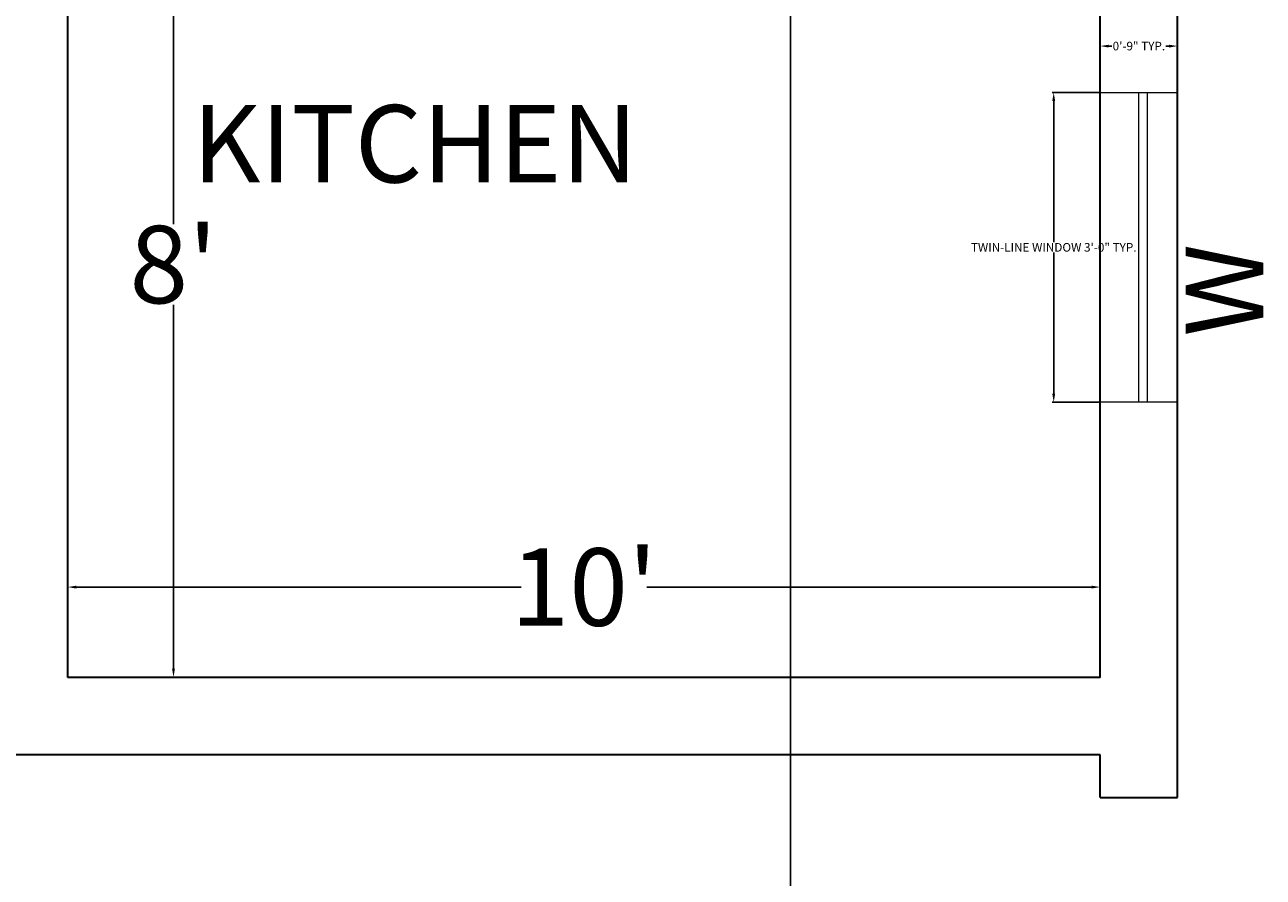
# Model space of a CAD drawing. Units: inches. Extents: x -2189 to 546, y 945 to 2684.
# Tile 6 of 10: x -492 to -348, y 2267 to 2366. Entities that reach past the tile are written whole.
import ezdxf

# ---------------------------------------------------------------- set-up
doc = ezdxf.new("R2010")
doc.units = ezdxf.units.IN
doc.header["$MEASUREMENT"] = 0
for name, color, linetype, lineweight in [('A-ANNO-DIMS', 2, 'Continuous', 13), ('A-ANNO-TEXT', 7, 'Continuous', 18), ('A-AREA-IDEN', 3, 'Continuous', 18), ('A-GLAZ', 4, 'Continuous', 18), ('A-WALL', 7, 'Continuous', 35)]:
    doc.layers.add(name, color=color, linetype=linetype, lineweight=lineweight)
doc.styles.get("Standard").update_dxf_attribs({"font": 'arial.ttf'})
doc.dimstyles.get("Standard").update_dxf_attribs({"dimtxt": 1, "dimasz": 1, "dimexe": 0.18, "dimexo": 0.0625, "dimgap": 0.09, "dimtad": 0, "dimtih": 1, "dimtoh": 1, "dimdec": 0, "dimzin": 0, "dimdsep": 46, "dimlunit": 3, "dimtxsty": 'Standard', "dimcen": 0.09, "dimadec": 0, "dimazin": 0, "dimtfac": 1, "dimtdec": 0, "dimtofl": 0, "dimtmove": 0, "dimatfit": 3, "dimfxl": 1, "dimtolj": 1, "dimtzin": 0, "dimarcsym": 0})

# ---------------------------------------------------------------- blocks, each defined once
blk = doc.blocks.new('*D70')
at = {"layer": 'A-ANNO-DIMS', "color": 0, "lineweight": -2, "transparency": 16777216}
for p, q in [((-486.72, 2386.17), (-474.31, 2386.17)), ((-474.49, 2385.17), (-474.49, 2342.86)), ((-474.49, 2291.17), (-474.49, 2333.49)), ((-486.72, 2290.17), (-474.31, 2290.17))]:
    blk.add_line(p, q, dxfattribs=at)
at = {"layer": 'A-ANNO-DIMS', "color": 0, "transparency": 16777216}
for points in [[(-474.66, 2385.17), (-474.33, 2385.17), (-474.49, 2386.17)], [(-474.66, 2291.17), (-474.33, 2291.17), (-474.49, 2290.17)]]:
    blk.add_solid(points, dxfattribs=at)
at = {"layer": 'Defpoints', "color": 0, "transparency": 16777216}
for p in [(-486.78, 2386.17), (-486.78, 2290.17), (-474.49, 2290.17)]:
    blk.add_point(p, dxfattribs=at)
at = {"layer": 'A-ANNO-DIMS', "color": 0, "transparency": 16777216, "insert": (-474.49, 2338.17), "char_height": 1, "attachment_point": 5}
blk.add_mtext("\\A1;{\\H9x;8'}", dxfattribs=at)
blk = doc.blocks.new('*D71')
at = {"layer": 'A-ANNO-DIMS', "color": 0, "lineweight": -2, "transparency": 16777216}
for p, q in [((-486.78, 2290.24), (-486.78, 2300.85)), ((-485.78, 2300.67), (-434.08, 2300.67)), ((-367.78, 2300.67), (-419.48, 2300.67)), ((-366.78, 2290.24), (-366.78, 2300.85))]:
    blk.add_line(p, q, dxfattribs=at)
at = {"layer": 'A-ANNO-DIMS', "color": 0, "transparency": 16777216}
for points in [[(-485.78, 2300.84), (-485.78, 2300.5), (-486.78, 2300.67)], [(-367.78, 2300.84), (-367.78, 2300.5), (-366.78, 2300.67)]]:
    blk.add_solid(points, dxfattribs=at)
at = {"layer": 'Defpoints', "color": 0, "transparency": 16777216}
for p in [(-366.78, 2300.67), (-486.78, 2290.17), (-366.78, 2290.17)]:
    blk.add_point(p, dxfattribs=at)
at = {"layer": 'A-ANNO-DIMS', "color": 0, "transparency": 16777216, "insert": (-426.78, 2300.67), "char_height": 1, "attachment_point": 5}
blk.add_mtext("\\A1;{\\H9x;10'}", dxfattribs=at)
blk = doc.blocks.new('WIN-36X9-TWINLINE')
for p, q in [((4.5, 0), (4.5, 36)), ((5.5, 0), (5.5, 36))]:
    blk.add_line(p, q)
blk.add_lwpolyline([(9, 0), (0, 0), (0, 36), (9, 36)], close=True)
blk = doc.blocks.new('*D93')
at = {"layer": 'A-ANNO-DIMS', "color": 0, "lineweight": -2, "transparency": 16777216}
for p, q in [((-366.84, 2358.17), (-372.36, 2358.17)), ((-372.18, 2357.17), (-372.18, 2340.78)), ((-372.18, 2323.17), (-372.18, 2339.56)), ((-366.84, 2322.17), (-372.36, 2322.17))]:
    blk.add_line(p, q, dxfattribs=at)
at = {"layer": 'A-ANNO-DIMS', "color": 0, "transparency": 16777216}
for points in [[(-372.35, 2357.17), (-372.01, 2357.17), (-372.18, 2358.17)], [(-372.35, 2323.17), (-372.01, 2323.17), (-372.18, 2322.17)]]:
    blk.add_solid(points, dxfattribs=at)
at = {"layer": 'Defpoints', "color": 0, "transparency": 16777216}
for p in [(-372.18, 2358.17), (-366.78, 2358.17), (-366.78, 2322.17)]:
    blk.add_point(p, dxfattribs=at)
at = {"layer": 'A-ANNO-DIMS', "color": 0, "transparency": 16777216, "insert": (-372.18, 2340.17), "char_height": 1, "attachment_point": 5}
blk.add_mtext('\\A1;TWIN-LINE WINDOW 3\'-0" TYP.', dxfattribs=at)
blk = doc.blocks.new('*D94')
at = {"layer": 'A-ANNO-DIMS', "color": 0, "lineweight": -2, "transparency": 16777216}
for p, q in [((-366.78, 2358.23), (-366.78, 2363.75)), ((-357.78, 2358.23), (-357.78, 2363.75)), ((-365.78, 2363.57), (-365.42, 2363.57)), ((-358.78, 2363.57), (-359.14, 2363.57))]:
    blk.add_line(p, q, dxfattribs=at)
at = {"layer": 'A-ANNO-DIMS', "color": 0, "transparency": 16777216}
for points in [[(-365.78, 2363.73), (-365.78, 2363.4), (-366.78, 2363.57)], [(-358.78, 2363.73), (-358.78, 2363.4), (-357.78, 2363.57)]]:
    blk.add_solid(points, dxfattribs=at)
at = {"layer": 'Defpoints', "color": 0, "transparency": 16777216}
for p in [(-357.78, 2363.57), (-366.78, 2358.17), (-357.78, 2358.17)]:
    blk.add_point(p, dxfattribs=at)
at = {"layer": 'A-ANNO-DIMS', "color": 0, "transparency": 16777216, "insert": (-362.28, 2363.57), "char_height": 1, "attachment_point": 5}
blk.add_mtext('\\A1;0\'-9" TYP.', dxfattribs=at)
blk = doc.blocks.new('*D104')
at = {"layer": 'A-ANNO-DIMS', "color": 0, "lineweight": -2, "transparency": 16777216}
for p, q in [((-493.78, 1873.24), (-493.78, 2683.65)), ((-492.78, 2683.47), (-449.69, 2683.47)), ((-403.78, 2683.47), (-446.86, 2683.47)), ((-402.78, 1873.24), (-402.78, 2683.65))]:
    blk.add_line(p, q, dxfattribs=at)
at = {"layer": 'A-ANNO-DIMS', "color": 0, "transparency": 16777216}
for points in [[(-492.78, 2683.64), (-492.78, 2683.31), (-493.78, 2683.47)], [(-403.78, 2683.64), (-403.78, 2683.31), (-402.78, 2683.47)]]:
    blk.add_solid(points, dxfattribs=at)
at = {"layer": 'Defpoints', "color": 0, "transparency": 16777216}
for p in [(-402.78, 2683.47), (-493.78, 1873.17), (-402.78, 1873.17)]:
    blk.add_point(p, dxfattribs=at)
at = {"layer": 'A-ANNO-DIMS', "color": 0, "transparency": 16777216, "insert": (-448.28, 2683.47), "char_height": 1, "attachment_point": 5}
blk.add_mtext('\\A1;7\'-7"', dxfattribs=at)

msp = doc.modelspace()

# ---------------------------------------------------------------- linework, layer by layer
at = {"layer": 'A-WALL'}
for p, q in [((-357.78, 2276.2), (-357.78, 2446.17)), ((-486.78, 2290.17), (-486.78, 2386.17)), ((-366.78, 2290.17), (-366.78, 2386.17)), ((-366.78, 2290.17), (-486.78, 2290.17)), ((-366.78, 2281.17), (-690.78, 2281.17)), ((-366.78, 2276.2), (-366.78, 2281.17)), ((-366.78, 2276.2), (-357.78, 2276.2))]:
    msp.add_line(p, q, dxfattribs=at)

# ---------------------------------------------------------------- block references
at = {"layer": 'A-GLAZ'}
msp.add_blockref('WIN-36X9-TWINLINE', (-366.78, 2322.17), dxfattribs=at)

# ---------------------------------------------------------------- texts
at = {"layer": 'A-ANNO-TEXT', "insert": (-356.83, 2329.79), "char_height": 9, "attachment_point": 1, "rotation": 90}
msp.add_mtext_dynamic_manual_height_columns('W', width=11.3125, gutter_width=1, heights=[0], dxfattribs=at)
at = {"layer": 'A-AREA-IDEN', "insert": (-472.3, 2356.71), "char_height": 9, "attachment_point": 1}
msp.add_mtext_dynamic_manual_height_columns('KITCHEN', width=69.371, gutter_width=1, heights=[0], dxfattribs=at)

# ---------------------------------------------------------------- dimensions: what is measured, and where the dimension line sits
at = {"layer": 'A-ANNO-DIMS'}
dim = msp.add_linear_dim(base=(-402.78, 2683.47), p1=(-493.78, 1873.17), p2=(-402.78, 1873.17), dimstyle='Standard', override={"dimdec": 1, "dimlfac": 1, "dimrnd": 0, "dimzin": 1, "dimdsep": 46, "dimlunit": 4, "dimfrac": 2}, dxfattribs=at)
dim.commit()
dim.dimension.update_dxf_attribs({"geometry": '*D104', "text_midpoint": (-448.28, 2683.47)})
for base, p1, p2, angle, text, override, picture, middle in [((-474.49, 2290.17), (-486.78, 2386.17), (-486.78, 2290.17), 90, '{\\H9x;<>}', {"dimclrd": 0, "dimclre": 0, "dimclrt": 0}, '*D70', (-474.49, 2338.17)), ((-372.18, 2358.17), (-366.78, 2322.17), (-366.78, 2358.17), 90, 'TWIN-LINE WINDOW <> TYP.', {"dimdec": 1, "dimlfac": 1, "dimrnd": 0, "dimzin": 1, "dimdsep": 46, "dimlunit": 4, "dimfrac": 2}, '*D93', (-372.18, 2340.17)), ((-366.78, 2300.67), (-486.78, 2290.17), (-366.78, 2290.17), 180, '{\\H9x;<>}', {"dimclrd": 0, "dimclre": 0, "dimclrt": 0}, '*D71', (-426.78, 2300.67))]:
    dim = msp.add_linear_dim(base=base, p1=p1, p2=p2, angle=angle, text=text, dimstyle='Standard', override=override, dxfattribs=at)
    dim.commit()
    dim.dimension.update_dxf_attribs({"geometry": picture, "text_midpoint": middle})
dim = msp.add_linear_dim(base=(-357.78, 2363.57), p1=(-366.78, 2358.17), p2=(-357.78, 2358.17), text='<> TYP.', dimstyle='Standard', override={"dimdec": 1, "dimlfac": 1, "dimrnd": 0, "dimzin": 1, "dimdsep": 46, "dimlunit": 4, "dimfrac": 2}, dxfattribs=at)
dim.commit()
dim.dimension.update_dxf_attribs({"geometry": '*D94', "text_midpoint": (-362.28, 2363.57)})

doc.saveas('drawing.dxf')
